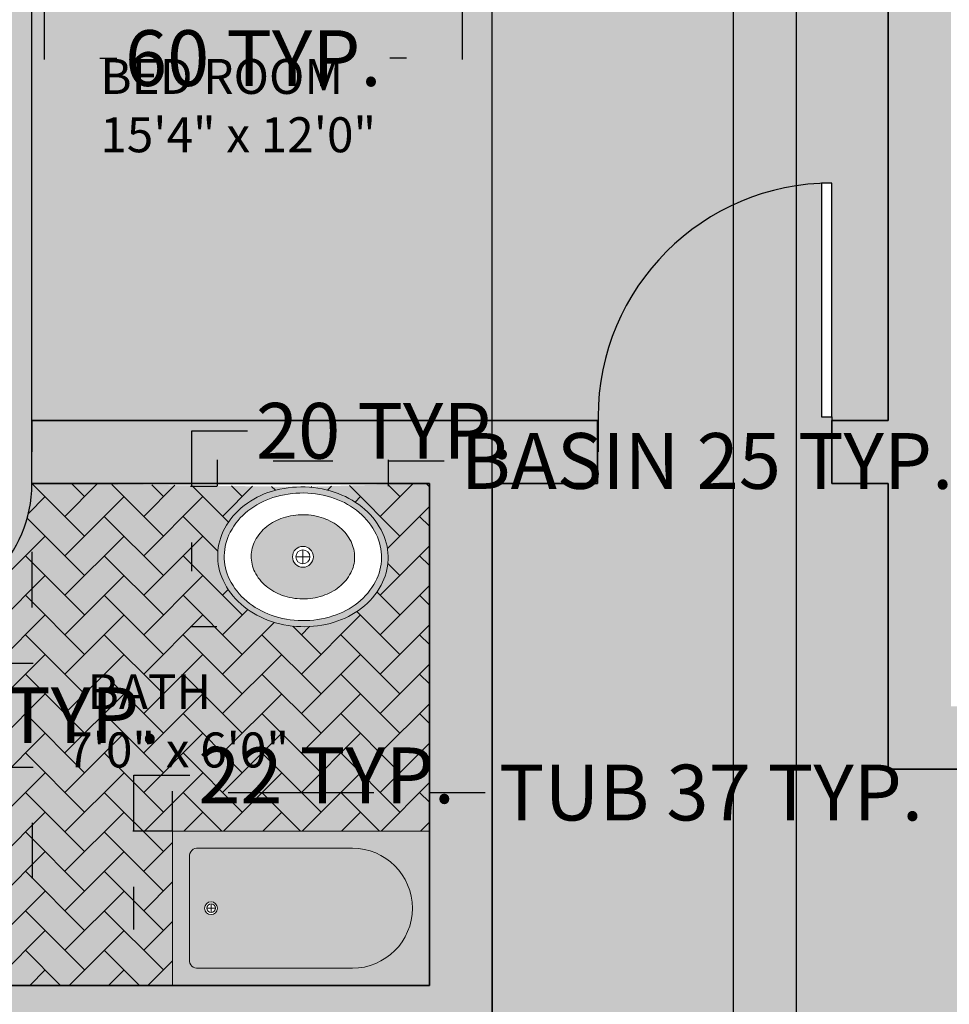
# Model space of a CAD drawing. Units: inches. Extents: x 389 to 971, y 148 to 870.
# Tile 10 of 14: x 537 to 670, y 558 to 699. Entities that reach past the tile are written whole.
import ezdxf

# ---------------------------------------------------------------- set-up
doc = ezdxf.new("R2010")
doc.units = ezdxf.units.IN
doc.header["$MEASUREMENT"] = 0
for name, color, linetype, lineweight in [('A-ANNO-DIMS', 2, 'Continuous', 18), ('A-AREA-IDEN', 7, 'Continuous', 18), ('A-DOOR', 4, 'Continuous', 25), ('A-FLOR-BASE-PATT', 8, 'Continuous', 13), ('A-FLOR-FIXT', 8, 'Continuous', 18), ('A-FLOR-FIXT-PATT', 9, 'Continuous', 13), ('A-FLOR-PATT', 9, 'Continuous', 13), ('A-WALL', 7, 'Continuous', 35)]:
    doc.layers.add(name, color=color, linetype=linetype, lineweight=lineweight)
doc.layers.add('A-WALL-PATT', color=18, linetype='Continuous', lineweight=13, true_color=0x000000)
doc.styles.get("Standard").update_dxf_attribs({"font": 'arial.ttf'})
doc.dimstyles.get("Standard").update_dxf_attribs({"dimtxt": 8, "dimasz": 8, "dimexe": 0.18, "dimexo": 0.0625, "dimgap": 0.09, "dimtad": 0, "dimtih": 1, "dimtoh": 1, "dimdec": 0, "dimzin": 0, "dimdsep": 46, "dimlunit": 3, "dimtxsty": 'Standard', "dimcen": 0.09, "dimadec": 0, "dimazin": 0, "dimtfac": 1, "dimtdec": 0, "dimtofl": 0, "dimtmove": 0, "dimatfit": 3, "dimfxl": 1, "dimtolj": 1, "dimtzin": 0, "dimarcsym": 0})

# ---------------------------------------------------------------- blocks, each defined once
blk = doc.blocks.new('*U4')
for p, q in [((0, 0), (0, 6)), ((24, 0), (24, 6))]:
    blk.add_line(p, q)
blk.add_lwpolyline([(0, 0), (0, -24), (1.75, -24), (1.75, 0)], close=True)
blk.add_arc((0, 0), 24, 270, 0)
blk = doc.blocks.new('*U3')
for p, q in [((0, 0), (0, -6)), ((-40, 0), (-40, -6))]:
    blk.add_line(p, q)
blk.add_lwpolyline([(0, 0), (0, 40), (-1.75, 40), (-1.75, 0)], close=True)
blk.add_arc((0, 0), 40, 90, 180)
blk = doc.blocks.new('Sink - Oval top')
for p, q in [((-1, 0), (1, 0)), ((0, 1), (0, -1))]:
    blk.add_line(p, q)
for points in [[(-12.23, 0.39, 0.117634), (-11.46, -3.36, 0.104469), (-8.88, -6.8, 0.090016), (-5.08, -9.07, 0.08192), (-0.32, -10.02, 0.08192), (4.49, -9.38, 0.090016), (8.42, -7.36, 0.104469), (11.22, -4.09, 0.117634), (12.23, -0.39, 0.117634), (11.46, 3.36, 0.104469), (8.88, 6.8, 0.090016), (5.08, 9.07, 0.08192), (0.32, 10.02, 0.08192), (-4.49, 9.38, 0.090016), (-8.42, 7.36, 0.104469), (-11.22, 4.09, 0.117634)], [(-11.29, 0.16, 0.118622), (-10.52, -3.25, 0.104678), (-8.07, -6.36, 0.089562), (-4.54, -8.37, 0.081185), (-0.13, -9.15, 0.081185), (4.3, -8.49, 0.089562), (7.89, -6.58, 0.104678), (10.42, -3.55, 0.118622), (11.29, -0.16, 0.118622), (10.52, 3.25, 0.104678), (8.07, 6.36, 0.089562), (4.54, 8.37, 0.081185), (0.13, 9.15, 0.081185), (-4.3, 8.49, 0.089562), (-7.89, 6.58, 0.104678), (-10.42, 3.55, 0.118622)], [(-7.42, 0.08, 0.118283), (-6.91, -2.17, 0.104607), (-5.29, -4.21, 0.089718), (-2.97, -5.53, 0.081436), (-0.07, -6.04, 0.081436), (2.84, -5.59, 0.089718), (5.2, -4.33, 0.104607), (6.86, -2.32, 0.118283), (7.42, -0.08, 0.118283), (6.91, 2.17, 0.104607), (5.29, 4.21, 0.089718), (2.97, 5.53, 0.081436), (0.07, 6.04, 0.081436), (-2.84, 5.59, 0.089718), (-5.2, 4.33, 0.104607), (-6.86, 2.32, 0.118283)]]:
    blk.add_lwpolyline(points, format="xyb", close=True)
for radius in [1.5, 1]:
    blk.add_circle((0, 0), radius)
blk = doc.blocks.new('Bath Tub - 26 x 60 in.')
for p, q in [((8, -18), (10, -18)), ((9, -17), (9, -19))]:
    blk.add_line(p, q)
blk.add_lwpolyline([(0, -36), (0, 0), (60, 0), (60, -36)], close=True)
for points in [[(6, -4), (42, -4)], [(4, -30), (4, -6)], [(42, -32), (6, -32)]]:
    blk.add_lwpolyline(points)
for radius in [1.5, 1]:
    blk.add_circle((9, -18), radius)
for centre, radius, start, end in [((5.75, -5.75), 1.77, 81.8699, 188.1301), ((42, -18), 14, 270, 90), ((5.75, -30.25), 1.77, 171.8699, 278.1301)]:
    blk.add_arc(centre, radius, start, end)
blk = doc.blocks.new('*D25')
at = {"layer": 'A-ANNO-DIMS', "color": 0, "lineweight": -2, "transparency": 16777216}
for p, q in [((540.09, 705.58), (540.09, 693.46)), ((600.09, 705.58), (600.09, 693.46)), ((548.09, 693.64), (550.51, 693.64)), ((592.09, 693.64), (589.67, 693.64))]:
    blk.add_line(p, q, dxfattribs=at)
at = {"layer": 'A-ANNO-DIMS', "color": 0, "transparency": 16777216}
for points in [[(548.09, 694.98), (548.09, 692.31), (540.09, 693.64)], [(592.09, 694.98), (592.09, 692.31), (600.09, 693.64)]]:
    blk.add_solid(points, dxfattribs=at)
at = {"layer": 'Defpoints', "color": 0, "transparency": 16777216}
for p in [(540.09, 705.64), (600.09, 705.64), (600.09, 693.64)]:
    blk.add_point(p, dxfattribs=at)
at = {"layer": 'A-ANNO-DIMS', "color": 0, "transparency": 16777216, "insert": (570.09, 693.64), "char_height": 8, "attachment_point": 5}
blk.add_mtext('\\A1;60 TYP.', dxfattribs=at)
blk = doc.blocks.new('*D27')
at = {"layer": 'A-ANNO-DIMS', "color": 0, "lineweight": -2, "transparency": 16777216}
for p, q in [((538.35, 614.84), (538.35, 622.84)), ((534.89, 606.84), (538.53, 606.84)), ((534.89, 591.95), (538.53, 591.95)), ((538.35, 583.95), (538.35, 575.95))]:
    blk.add_line(p, q, dxfattribs=at)
at = {"layer": 'A-ANNO-DIMS', "color": 0, "transparency": 16777216}
for points in [[(537.01, 614.84), (539.68, 614.84), (538.35, 606.84)], [(537.01, 583.95), (539.68, 583.95), (538.35, 591.95)]]:
    blk.add_solid(points, dxfattribs=at)
at = {"layer": 'Defpoints', "color": 0, "transparency": 16777216}
for p in [(534.83, 606.84), (538.35, 606.84), (534.83, 591.95)]:
    blk.add_point(p, dxfattribs=at)
at = {"layer": 'A-ANNO-DIMS', "color": 0, "transparency": 16777216, "insert": (538.35, 599.39), "char_height": 8, "attachment_point": 5}
blk.add_mtext('\\A1;15 TYP.', dxfattribs=at)
blk = doc.blocks.new('*D28')
at = {"layer": 'A-ANNO-DIMS', "color": 0, "lineweight": -2, "transparency": 16777216}
for p, q in [((564.95, 632.24), (564.95, 636.04)), ((572.95, 635.86), (581.5, 635.86)), ((589.5, 632.24), (589.5, 636.04)), ((589.5, 635.86), (597.5, 635.86))]:
    blk.add_line(p, q, dxfattribs=at)
at = {"layer": 'A-ANNO-DIMS', "color": 0, "transparency": 16777216}
for points in [[(572.95, 637.2), (572.95, 634.53), (564.95, 635.86)], [(581.5, 637.2), (581.5, 634.53), (589.5, 635.86)]]:
    blk.add_solid(points, dxfattribs=at)
at = {"layer": 'Defpoints', "color": 0, "transparency": 16777216}
for p in [(589.5, 635.86), (564.95, 632.18), (589.5, 632.18)]:
    blk.add_point(p, dxfattribs=at)
at = {"layer": 'A-ANNO-DIMS', "color": 0, "transparency": 16777216, "insert": (635.2, 635.86), "char_height": 8, "attachment_point": 5}
blk.add_mtext('\\A1;BASIN 25 TYP.', dxfattribs=at)
blk = doc.blocks.new('*D29')
at = {"layer": 'A-ANNO-DIMS', "color": 0, "lineweight": -2, "transparency": 16777216}
for p, q in [((561.26, 632.18), (561.26, 640.18)), ((561.26, 640.18), (569.26, 640.18)), ((564.88, 632.18), (561.08, 632.18)), ((561.26, 620.05), (561.26, 624.18)), ((564.88, 612.05), (561.08, 612.05))]:
    blk.add_line(p, q, dxfattribs=at)
at = {"layer": 'A-ANNO-DIMS', "color": 0, "transparency": 16777216}
for points in [[(559.93, 624.18), (562.6, 624.18), (561.26, 632.18)], [(559.93, 620.05), (562.6, 620.05), (561.26, 612.05)]]:
    blk.add_solid(points, dxfattribs=at)
at = {"layer": 'Defpoints', "color": 0, "transparency": 16777216}
for p in [(561.26, 632.18), (564.95, 632.18), (564.95, 612.05)]:
    blk.add_point(p, dxfattribs=at)
at = {"layer": 'A-ANNO-DIMS', "color": 0, "transparency": 16777216, "insert": (588.89, 640.18), "char_height": 8, "attachment_point": 5}
blk.add_mtext('\\A1;20 TYP.', dxfattribs=at)
blk = doc.blocks.new('*D30')
at = {"layer": 'A-ANNO-DIMS', "color": 0, "lineweight": -2, "transparency": 16777216}
for p, q in [((558.51, 582.83), (558.51, 588.48)), ((566.51, 588.3), (587.39, 588.3)), ((595.39, 582.83), (595.39, 588.48)), ((595.39, 588.3), (603.39, 588.3))]:
    blk.add_line(p, q, dxfattribs=at)
at = {"layer": 'A-ANNO-DIMS', "color": 0, "transparency": 16777216}
for points in [[(566.51, 589.64), (566.51, 586.97), (558.51, 588.3)], [(587.39, 589.64), (587.39, 586.97), (595.39, 588.3)]]:
    blk.add_solid(points, dxfattribs=at)
at = {"layer": 'Defpoints', "color": 0, "transparency": 16777216}
for p in [(595.39, 588.3), (558.51, 582.77), (595.39, 582.77)]:
    blk.add_point(p, dxfattribs=at)
at = {"layer": 'A-ANNO-DIMS', "color": 0, "transparency": 16777216, "insert": (635.78, 588.3), "char_height": 8, "attachment_point": 5}
blk.add_mtext('\\A1;TUB 37 TYP.', dxfattribs=at)
blk = doc.blocks.new('*D31')
at = {"layer": 'A-ANNO-DIMS', "color": 0, "lineweight": -2, "transparency": 16777216}
for p, q in [((552.98, 582.77), (552.98, 590.77)), ((552.98, 590.77), (560.98, 590.77)), ((558.45, 582.77), (552.8, 582.77)), ((552.98, 568.64), (552.98, 574.77)), ((558.45, 560.64), (552.8, 560.64))]:
    blk.add_line(p, q, dxfattribs=at)
at = {"layer": 'A-ANNO-DIMS', "color": 0, "transparency": 16777216}
for points in [[(551.64, 574.77), (554.31, 574.77), (552.98, 582.77)], [(551.64, 568.64), (554.31, 568.64), (552.98, 560.64)]]:
    blk.add_solid(points, dxfattribs=at)
at = {"layer": 'Defpoints', "color": 0, "transparency": 16777216}
for p in [(552.98, 582.77), (558.51, 582.77), (558.51, 560.64)]:
    blk.add_point(p, dxfattribs=at)
at = {"layer": 'A-ANNO-DIMS', "color": 0, "transparency": 16777216, "insert": (580.61, 590.77), "char_height": 8, "attachment_point": 5}
blk.add_mtext('\\A1;22 TYP.', dxfattribs=at)
blk = doc.blocks.new('*D49')
at = {"layer": 'A-ANNO-DIMS', "color": 0, "lineweight": -2, "transparency": 16777216}
for p, q in [((519.98, 632.71), (519.98, 865.15)), ((527.98, 864.97), (530.32, 864.97)), ((538.32, 632.71), (538.32, 865.15)), ((538.32, 864.97), (546.32, 864.97))]:
    blk.add_line(p, q, dxfattribs=at)
at = {"layer": 'A-ANNO-DIMS', "color": 0, "transparency": 16777216}
for points in [[(527.98, 866.3), (527.98, 863.64), (519.98, 864.97)], [(530.32, 866.3), (530.32, 863.64), (538.32, 864.97)]]:
    blk.add_solid(points, dxfattribs=at)
at = {"layer": 'Defpoints', "color": 0, "transparency": 16777216}
for p in [(538.32, 864.97), (519.98, 632.64), (538.32, 632.64)]:
    blk.add_point(p, dxfattribs=at)
at = {"layer": 'A-ANNO-DIMS', "color": 0, "transparency": 16777216, "insert": (559.52, 864.97), "char_height": 8, "attachment_point": 5}
blk.add_mtext('\\A1;18.34', dxfattribs=at)
blk = doc.blocks.new('*D51')
at = {"layer": 'A-ANNO-DIMS', "color": 0, "lineweight": -2, "transparency": 16777216}
for p, q in [((596.39, 864.97), (588.39, 864.97)), ((604.39, 354.78), (604.39, 865.15)), ((639.03, 354.78), (639.03, 865.15)), ((647.03, 864.97), (655.03, 864.97))]:
    blk.add_line(p, q, dxfattribs=at)
at = {"layer": 'A-ANNO-DIMS', "color": 0, "transparency": 16777216}
for points in [[(596.39, 866.3), (596.39, 863.64), (604.39, 864.97)], [(647.03, 866.3), (647.03, 863.64), (639.03, 864.97)]]:
    blk.add_solid(points, dxfattribs=at)
at = {"layer": 'Defpoints', "color": 0, "transparency": 16777216}
for p in [(639.03, 864.97), (604.39, 354.72), (639.03, 354.72)]:
    blk.add_point(p, dxfattribs=at)
at = {"layer": 'A-ANNO-DIMS', "color": 0, "transparency": 16777216, "insert": (621.71, 864.97), "char_height": 8, "attachment_point": 5}
blk.add_mtext('\\A1;34.64', dxfattribs=at)
blk = doc.blocks.new('*D52')
at = {"layer": 'A-ANNO-DIMS', "color": 0, "lineweight": -2, "transparency": 16777216}
for p, q in [((640.06, 864.97), (632.06, 864.97)), ((648.06, 388.98), (648.06, 865.15)), ((690.22, 388.98), (690.22, 865.15)), ((698.22, 864.97), (706.22, 864.97))]:
    blk.add_line(p, q, dxfattribs=at)
at = {"layer": 'A-ANNO-DIMS', "color": 0, "transparency": 16777216}
for points in [[(640.06, 866.3), (640.06, 863.64), (648.06, 864.97)], [(698.22, 866.3), (698.22, 863.64), (690.22, 864.97)]]:
    blk.add_solid(points, dxfattribs=at)
at = {"layer": 'Defpoints', "color": 0, "transparency": 16777216}
for p in [(690.22, 864.97), (648.06, 388.92), (690.22, 388.92)]:
    blk.add_point(p, dxfattribs=at)
at = {"layer": 'A-ANNO-DIMS', "color": 0, "transparency": 16777216, "insert": (669.14, 864.97), "char_height": 8, "attachment_point": 5}
blk.add_mtext('\\A1;42.155', dxfattribs=at)

msp = doc.modelspace()

# ---------------------------------------------------------------- hatches: boundary and pattern name
at = {"layer": 'A-FLOR-BASE-PATT'}
h = msp.add_hatch(color=256, dxfattribs=at)
h.dxf.hatch_style = 1
h.paths.add_polyline_path([(651.6417, 675.6801), (651.6417, 675.7122), (653.109, 675.7122), (653.109, 641.6445), (661.216, 641.6445), (661.216, 785.6445), (616.7487, 785.6445), (616.7487, 768.9039), (600.0901, 768.9039), (600.0901, 705.6445), (540.0901, 705.6445), (540.0901, 768.9039), (523.3494, 768.9039), (523.3494, 785.6445), (477.216, 785.6445), (477.216, 777.4428), (477.216, 728.9805), (477.216, 699.1491), (477.216, 651.2738), (477.216, 641.6445), (519.983, 641.6445), (519.983, 632.5593), (521.3203, 632.5593), (521.3203, 614.2674, 0.39433689), (538.3235, 632.6445), (538.3237, 632.6445), (538.3237, 637.1445), (538.3237, 641.6445), (619.5719, 641.6445), (619.5719, 642.1751, -0.40145271)])
h.paths.add_polyline_path([(546.1308, 677.2872), (587.0907, 677.2872), (587.0907, 696.0138), (546.1308, 696.0138)], flags=24)
h = msp.add_hatch(color=256, dxfattribs=at)
h.dxf.hatch_style = 1
h.paths.add_polyline_path([(634.6594, 428.4021), (634.6594, 427.0792), (634.6305, 427.0792, -0.40145271), (604.4225, 398.1652), (604.0817, 398.1199, -0.40145271), (632.0195, 371.3788), (632.0462, 371.3788), (632.0462, 370.1554), (604.387, 370.1554), (604.387, 366.7191), (640.0296, 366.7191), (640.0296, 321.4969, 1), (647.061, 321.4969), (647.061, 412.9189), (690.216, 412.9189), (690.216, 416.0006), (694.716, 416.0006), (702.2145, 416.0006, 0.39601219), (737.1392, 448.8066), (702.2145, 448.8066), (702.2145, 450.9936), (694.716, 450.9936), (690.216, 450.9936), (690.216, 466.6012), (708.7881, 466.6012), (708.7881, 462.1012), (784.6145, 462.1012), (784.6145, 466.6012), (794.216, 466.6012), (794.216, 591.6445), (708.5171, 591.6445), (708.5171, 596.1445), (708.5171, 602.9755, 0.39601219), (678.6314, 634.7912), (678.6314, 602.9755), (676.6391, 602.9755), (676.6391, 596.1445), (676.6391, 591.6445), (661.216, 591.6445), (661.216, 632.6445), (653.109, 632.6445), (653.109, 641.6445), (653.109, 642.1751), (651.6417, 642.1751), (651.6417, 675.6801, 0.40145271), (619.5719, 642.1751), (619.5719, 637.1445), (619.5147, 632.6445), (604.387, 632.6445), (604.387, 545.7317), (595.3894, 545.7317), (595.3894, 544.4199), (565.4338, 544.4199, 0.40145271), (595.3894, 515.7475), (599.887, 515.7475), (604.387, 515.7271), (604.387, 428.4021)])
h.paths.add_polyline_path([(721.8003, 493.9292), (725.0899, 493.9292), (725.0899, 493.075), (751.4065, 493.075), (751.4065, 493.9292), (754.6961, 493.9292), (754.6961, 479.6744, -0.26666697), (721.8003, 479.6744)], flags=16)
h.paths.add_polyline_path([(720.6421, 516.0583), (720.6421, 545.0393), (753.5806, 545.0393), (753.5806, 516.0583)], flags=16)
h.paths.add_polyline_path([(722.6421, 518.0583), (722.6421, 543.0393), (751.5806, 543.0393), (751.5806, 518.0583)], flags=0)
h.paths.add_polyline_path([(763.7396, 488.5801), (763.7822, 488.1156), (764.1436, 488.1761)], flags=16)
h.paths.add_polyline_path([(777.9011, 479.7417), (778.0475, 480.1886), (777.4745, 480.275)], flags=16)
h.paths.add_polyline_path([(762.3329, 503.5919), (762.3329, 507.1718), (763.2624, 507.1718), (763.2624, 550.1306), (762.3329, 550.1306), (762.3329, 553.7105), (777.8458, 553.7105, -0.19047621), (777.8458, 503.5919)], flags=16)
h.paths.add_polyline_path([(721.6097, 567.2898), (721.6097, 581.7362, -0.26666697), (754.9475, 581.7362), (754.9475, 567.2898), (751.6137, 567.2898), (751.6137, 568.1555), (724.9435, 568.1555), (724.9435, 567.2898)], flags=16)
h.paths.add_polyline_path([(774.6347, 521.4914), (774.6347, 535.811), (778.6837, 535.811, -0.04962821), (778.6837, 521.4914)], flags=0)
h.paths.add_polyline_path([(764.6624, 576.8996), (764.7454, 576.4742), (765.0717, 576.4903)], flags=16)
h.paths.add_polyline_path([(777.2772, 570.3652), (777.4444, 570.8756), (776.7899, 570.9743)], flags=16)
h.paths.add_polyline_path([(644.2892, 516.9956), (685.2491, 516.9956), (685.2491, 535.7223), (644.2892, 535.7223)], flags=24)
h = msp.add_hatch(color=256, dxfattribs=at)
h.dxf.hatch_style = 1
h.paths.add_polyline_path([(558.5088, 560.6445), (558.5088, 582.7714), (595.387, 582.7714), (595.387, 632.6445), (577.0646, 632.1376, -0.09003216), (582.3048, 631.1863, -0.09001579), (586.1007, 628.9176, -0.10446928), (588.6866, 625.476, -0.11763426), (589.4557, 621.7198, -0.11763426), (588.4463, 618.021, -0.10446928), (585.6443, 614.753, -0.09001579), (581.7102, 612.7333, -0.08191995), (576.8993, 612.0982, -0.08191995), (572.1392, 613.0417, -0.09001579), (568.3432, 615.3105, -0.10446928), (565.7574, 618.7521, -0.11763426), (564.9883, 622.5082, -0.11763426), (565.9976, 626.207, -0.10446928), (568.7997, 629.475, -0.09001579), (572.7338, 631.4947, -0.07381843), (577.0646, 632.1376), (538.3237, 632.6445), (538.3237, 632.5593, -0.39299579), (521.3203, 614.2674), (521.3203, 614.2186), (519.983, 614.2186), (519.983, 632.6445), (511.387, 632.6445), (511.387, 613.354), (511.387, 606.8427), (517.062, 606.8427), (517.062, 602.2317), (521.3182, 603.6504, -0.50132349), (534.6979, 600.1353, -0.13289091), (534.6979, 598.6532, -0.50131678), (521.3183, 595.1379), (517.062, 596.5567), (517.062, 594.4286), (518.1261, 594.4286), (518.1261, 592.3005), (517.062, 592.3005), (517.062, 591.9458), (511.387, 591.9458), (511.387, 585.4344), (511.387, 560.6445)])
h.paths.add_polyline_path([(541.6656, 589.1356), (574.8272, 589.1356), (574.8272, 607.8622), (541.6656, 607.8622)], flags=24)
at = {"layer": 'A-FLOR-FIXT-PATT'}
h = msp.add_hatch(color=256, dxfattribs=at)
h.dxf.hatch_style = 1
h.paths.add_polyline_path([(572.6843, 613.7471, 0.0811847), (577.093, 612.9625, 0.0811847), (581.5221, 613.6225, 0.08956207), (585.1114, 615.5305, 0.10467817), (587.642, 618.5658, 0.1186217), (588.5083, 621.955, 0.1186217), (587.7379, 625.3672, 0.10467817), (585.2938, 628.4726, 0.08956207), (581.7597, 630.481, 0.0811847), (577.351, 631.2655, 0.0811847), (572.9219, 630.6056, 0.08956207), (569.3326, 628.6976, 0.10467817), (566.8019, 625.6622, 0.1186217), (565.9357, 622.2731, 0.1186217), (566.7061, 618.8609, 0.10467817), (569.1502, 615.7554, 0.08956207)], flags=16)
h.paths.add_polyline_path([(571.9272, 617.904, -0.10460746), (570.3149, 619.9466, -0.11828257), (569.8015, 622.197, -0.11828257), (570.3651, 624.4354, -0.10460746), (572.0227, 626.4414, -0.08971796), (574.3798, 627.7071, -0.08143608), (577.2895, 628.1508, -0.08143608), (580.1886, 627.6422, -0.08971796), (582.5168, 626.324, -0.10460746), (584.1291, 624.2815, -0.11828257), (584.6424, 622.031, -0.11828257), (584.0789, 619.7926, -0.10460746), (582.4213, 617.7867, -0.08971796), (580.0642, 616.5209, -0.08143608), (577.1545, 616.0772, -0.08143608), (574.2554, 616.5859, -0.08971796)], flags=0)
h.paths.add_polyline_path([(572.1392, 613.0417, 0.08191995), (576.8993, 612.0982, 0.08191995), (581.7102, 612.7333, 0.09001579), (585.6443, 614.753, 0.10446928), (588.4463, 618.021, 0.11763426), (589.4557, 621.7198, 0.11763426), (588.6866, 625.476, 0.10446928), (586.1007, 628.9176, 0.09001579), (582.3048, 631.1863, 0.08191995), (577.5447, 632.1299, 0.08191995), (572.7338, 631.4947, 0.09001579), (568.7997, 629.475, 0.10446928), (565.9976, 626.207, 0.11763426), (564.9883, 622.5082, 0.11763426), (565.7574, 618.7521, 0.10446928), (568.3432, 615.3105, 0.09001579)])
h.paths.add_polyline_path([(575.722, 622.114, -1), (578.722, 622.114, -1)], flags=0)
h = msp.add_hatch(color=256, dxfattribs=at)
h.dxf.hatch_style = 1
h.paths.add_polyline_path([(582.4213, 617.7867, 0.10460746), (584.0789, 619.7926, 0.11828257), (584.6424, 622.031, 0.11828257), (584.1291, 624.2815, 0.10460746), (582.5168, 626.324, 0.08971796), (580.1886, 627.6422, 0.08143608), (577.2895, 628.1508, 0.08143608), (574.3798, 627.7071, 0.08971796), (572.0227, 626.4414, 0.10460746), (570.3651, 624.4354, 0.11828257), (569.8015, 622.197, 0.11828257), (570.3149, 619.9466, 0.10460746), (571.9272, 617.904, 0.08971796), (574.2554, 616.5859, 0.08143608), (577.1545, 616.0772, 0.08143608), (580.0642, 616.5209, 0.08971796)])
h.paths.add_polyline_path([(575.722, 622.114, -1), (578.722, 622.114, -1)], flags=16)
h.paths.add_polyline_path([(576.222, 622.114, -1), (578.222, 622.114, -1)], flags=0)
h = msp.add_hatch(color=256, dxfattribs=at)
h.dxf.hatch_style = 1
h.paths.add_polyline_path([(584.3236, 563.1031, 1), (584.3236, 580.3129), (562.1967, 580.3129, 0.50000012), (560.9674, 579.0836), (560.9674, 564.3323, 0.50000012), (562.1967, 563.1031)], flags=16)
h.paths.add_polyline_path([(595.387, 560.6445), (595.387, 582.7714), (558.5088, 582.7714), (558.5088, 560.6445)])
h.paths.add_polyline_path([(563.1186, 571.708, -1), (564.9625, 571.708, -1)], flags=0)
h.paths.add_polyline_path([(563.4259, 571.708, -1), (564.6552, 571.708, -1)], flags=0)
h = msp.add_hatch(color=256, dxfattribs=at)
h.dxf.hatch_style = 1
h.paths.add_polyline_path([(584.3236, 563.1031, 1), (584.3236, 580.3129), (562.1967, 580.3129, 0.50000012), (560.9674, 579.0836), (560.9674, 564.3323, 0.50000012), (562.1967, 563.1031)], flags=16)
h.paths.add_polyline_path([(595.387, 560.6445), (595.387, 582.7714), (558.5088, 582.7714), (558.5088, 560.6445)])
h.paths.add_polyline_path([(563.1186, 571.708, -1), (564.9625, 571.708, -1)], flags=0)
h = msp.add_hatch(color=256, dxfattribs=at)
h.dxf.hatch_style = 1
h.paths.add_polyline_path([(595.387, 582.7714), (558.5088, 582.7714), (558.5088, 560.6445), (595.387, 560.6445)])
h.paths.add_polyline_path([(584.3236, 563.1031), (562.1967, 563.1031, -0.50000012), (560.9674, 564.3323), (560.9674, 579.0836, -0.50000012), (562.1967, 580.3129), (584.3236, 580.3129, -1)], flags=16)
h.paths.add_polyline_path([(564.9625, 571.708, -1), (563.1186, 571.708, -1)], flags=0)
h.paths.add_polyline_path([(564.6552, 571.708, -1), (563.4259, 571.708, -1)], flags=0)
h = msp.add_hatch(color=256, dxfattribs=at)
h.dxf.hatch_style = 1
h.paths.add_polyline_path([(584.3236, 580.3129), (562.1967, 580.3129, 0.50000012), (560.9674, 579.0836), (560.9674, 564.3323, 0.50000012), (562.1967, 563.1031), (584.3236, 563.1031, 1)])
h.paths.add_polyline_path([(563.1186, 571.708, -1), (564.9625, 571.708, -1)], flags=16)
h.paths.add_polyline_path([(563.4259, 571.708, -1), (564.6552, 571.708, -1)], flags=0)
at = {"layer": 'A-FLOR-PATT'}
h = msp.add_hatch(dxfattribs=at)
h.set_pattern_fill('AR-HBONE', color=256)
h.paths.add_polyline_path([(521.3183, 595.1379), (517.062, 596.5567), (517.062, 594.4286), (518.1261, 594.4286), (518.1261, 592.3005), (517.062, 592.3005), (517.062, 591.9458), (511.387, 591.9458), (511.387, 585.4344), (511.387, 560.6445), (558.5088, 560.6445), (558.5088, 582.7714), (595.387, 582.7714), (595.387, 632.6445), (577.0646, 632.1376, -0.09003216), (582.3048, 631.1863, -0.09001579), (586.1007, 628.9176, -0.10446928), (588.6866, 625.476, -0.11763426), (589.4557, 621.7198, -0.11763426), (588.4463, 618.021, -0.10446928), (585.6443, 614.753, -0.09001579), (581.7102, 612.7333, -0.08191995), (576.8993, 612.0982, -0.08191995), (572.1392, 613.0417, -0.09001579), (568.3432, 615.3105, -0.10446928), (565.7574, 618.7521, -0.11763426), (564.9883, 622.5082, -0.11763426), (565.9976, 626.207, -0.10446928), (568.7997, 629.475, -0.09001579), (572.7338, 631.4947, -0.07381843), (577.0646, 632.1376), (538.3237, 632.6445), (538.3237, 632.5593, -0.39299579), (521.3203, 614.2674), (521.3203, 614.2186), (519.983, 614.2186), (519.983, 632.6445), (511.387, 632.6445), (511.387, 613.354), (511.387, 606.8427), (517.062, 606.8427), (517.062, 602.2317), (521.3182, 603.6504, -0.50132349), (534.6979, 600.1353, -0.13289091), (534.6979, 598.6532, -0.50131678)])
h.paths.add_polyline_path([(541.6656, 589.1356), (574.8272, 589.1356), (574.8272, 607.8622), (541.6656, 607.8622)], flags=24)
at = {"layer": 'A-WALL-PATT'}
h = msp.add_hatch(color=256, dxfattribs=at)
h.dxf.hatch_style = 1
h.paths.add_polyline_path([(661.216, 785.6445), (661.216, 641.6445), (653.109, 641.6445), (653.109, 637.1445), (653.109, 632.6445), (661.216, 632.6445), (661.216, 591.6445), (676.6391, 591.6445), (676.6391, 600.6445), (670.216, 600.6445), (670.216, 785.6445), (685.2392, 785.6445), (685.2392, 794.6445), (662.4125, 794.6445), (606.2724, 794.6445), (606.2724, 785.6445), (616.7487, 785.6445)])
h = msp.add_hatch(color=256, dxfattribs=at)
h.dxf.hatch_style = 1
h.paths.add_polyline_path([(538.3237, 641.6445), (538.3237, 637.1445), (538.3237, 632.6445), (595.387, 632.6445), (595.387, 560.6445), (558.5088, 560.6445), (511.387, 560.6445), (511.387, 585.4344), (502.387, 585.4344), (502.387, 560.6445), (468.216, 560.6445), (468.216, 543.0462), (477.216, 543.0462), (477.216, 551.6445), (595.387, 551.6445), (595.387, 545.7317), (595.3894, 545.7317), (599.887, 545.7317), (604.387, 545.7317), (604.387, 632.6445), (619.5147, 632.6445), (619.5147, 641.6445)])

# ---------------------------------------------------------------- linework, layer by layer
at = {"layer": 'A-WALL'}
for p, q in [((661.216, 785.6445), (661.216, 641.6445)), ((619.5147, 641.6445), (538.3237, 641.6445)), ((538.3237, 637.1445), (538.3237, 641.6445)), ((619.5147, 641.6445), (619.5147, 632.6445)), ((661.216, 641.6445), (653.109, 641.6445)), ((653.109, 641.6445), (653.109, 632.6445)), ((595.387, 632.6445), (538.3237, 632.6445)), ((595.387, 632.6445), (595.387, 560.6445)), ((619.5147, 632.6445), (604.387, 632.6445)), ((604.387, 632.6445), (604.387, 545.7317)), ((661.216, 632.6445), (653.109, 632.6445)), ((661.216, 632.6445), (661.216, 591.6445)), ((676.6391, 591.6445), (661.216, 591.6445)), ((595.387, 560.6445), (511.387, 560.6445))]:
    msp.add_line(p, q, dxfattribs=at)

# ---------------------------------------------------------------- block references
at = {"layer": 'A-DOOR'}
for name, p, xscale, yscale, zscale in [('*U3', (653.109, 642.1751), 0.8384273000073651, 0.8384273000073651, 0.8384273000073651), ('*U4', (519.983, 632.5593), 0.7641975514951928, 0.7641975514951928, 0.7641975514951928)]:
    msp.add_blockref(name, p, dxfattribs=dict(at, xscale=xscale, yscale=yscale, zscale=zscale))
at = {"layer": 'A-FLOR-FIXT'}
msp.add_blockref('Sink - Oval top', (577.222, 622.114), dxfattribs=at)
at = {"layer": 'A-FLOR-FIXT', "xscale": 0.6146362971528592, "yscale": 0.6146362971528592, "zscale": 0.6146362971528592}
msp.add_blockref('Bath Tub - 26 x 60 in.', (558.5088, 582.7714), dxfattribs=at)

# ---------------------------------------------------------------- texts
at = {"layer": 'A-AREA-IDEN', "char_height": 5.018573, "attachment_point": 1}
for s, insert in [('BED ROOM\\P15\'4" x 12\'0"', (548.1488, 693.5199)), ('  BATH\\P7\'0" x 6\'0"', (543.2523, 605.2794))]:
    msp.add_mtext_dynamic_manual_height_columns(s, width=113.900213, gutter_width=25.0929, heights=[0], dxfattribs=dict(at, insert=insert))

# ---------------------------------------------------------------- dimensions: what is measured, and where the dimension line sits
at = {"layer": 'A-ANNO-DIMS'}
for base, p1, p2, override, picture, middle in [((538.3237, 864.9695), (519.983, 632.6445), (538.3237, 632.6445), {"dimdec": 2, "dimlfac": 1, "dimrnd": 0, "dimzin": 0, "dimdsep": 46, "dimlunit": 2}, '*D49', (559.5188, 864.9695)), ((639.0296, 864.9695), (604.387, 354.7191), (639.0296, 354.7191), {"dimdec": 2, "dimlfac": 1, "dimrnd": 0, "dimzin": 0, "dimdsep": 46, "dimlunit": 2}, '*D51', (621.7083, 864.9695)), ((690.216, 864.9695), (648.061, 388.9189), (690.216, 388.9189), {"dimdec": 3, "dimlfac": 1, "dimrnd": 0, "dimzin": 0, "dimdsep": 46, "dimlunit": 2}, '*D52', (669.1385, 864.9695))]:
    dim = msp.add_linear_dim(base=base, p1=p1, p2=p2, dimstyle='Standard', override=override, dxfattribs=at)
    dim.commit()
    dim.dimension.update_dxf_attribs({"geometry": picture, "text_midpoint": middle})
for base, p1, p2, text, picture, middle in [((600.0901, 693.6445), (540.0901, 705.6445), (600.0901, 705.6445), '<> TYP.', '*D25', (570.0901, 693.6445)), ((589.4974, 635.865), (564.9465, 632.1823), (589.4974, 632.1823), 'BASIN <> TYP.', '*D28', (635.2027, 635.865)), ((595.387, 588.3031), (558.5088, 582.7714), (595.387, 582.7714), 'TUB <> TYP.', '*D30', (635.7771, 588.3031))]:
    dim = msp.add_linear_dim(base=base, p1=p1, p2=p2, text=text, dimstyle='Standard', override={"dimdec": 0, "dimlfac": 1, "dimrnd": 0, "dimzin": 0, "dimdsep": 46, "dimlunit": 2}, dxfattribs=at)
    dim.commit()
    dim.dimension.update_dxf_attribs({"geometry": picture, "text_midpoint": middle})
for base, p1, p2, picture, middle in [((561.2639, 632.1823), (564.9465, 612.0457), (564.9465, 632.1823), '*D29', (588.8928, 640.1823)), ((538.3455, 606.8427), (534.8292, 591.9458), (534.8292, 606.8427), '*D27', (538.3455, 599.3942)), ((552.9771, 582.7714), (558.5088, 560.6445), (558.5088, 582.7714), '*D31', (580.606, 590.7714))]:
    dim = msp.add_linear_dim(base=base, p1=p1, p2=p2, angle=90, text='<> TYP.', dimstyle='Standard', override={"dimdec": 0, "dimlfac": 1, "dimrnd": 0, "dimzin": 0, "dimdsep": 46, "dimlunit": 2}, dxfattribs=at)
    dim.commit()
    dim.dimension.update_dxf_attribs({"geometry": picture, "text_midpoint": middle})

doc.saveas('drawing.dxf')
